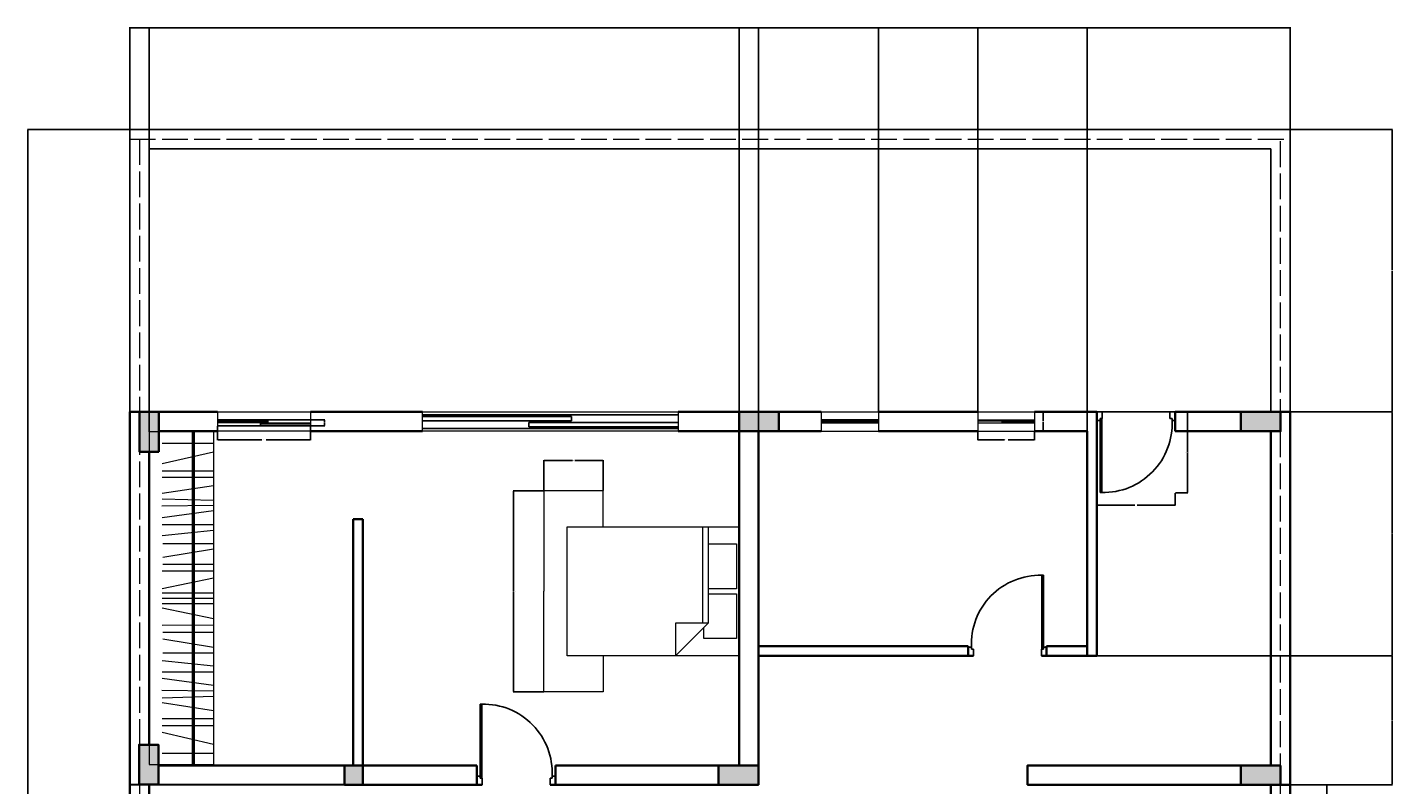
# Model space of a CAD drawing. Units: inches. Extents: x 2711 to 4246, y 540 to 1583.
# Tile 4 of 7: x 2716 to 3351, y 1230 to 1583. Entities that reach past the tile are written whole.
import ezdxf

# ---------------------------------------------------------------- set-up
doc = ezdxf.new("R2010")
doc.units = ezdxf.units.IN
doc.linetypes.add('ACAD_ISO02W100', pattern=[15, 12, -3])
for name, color, linetype, lineweight in [('A-ANNO-DIMS', 2, 'Continuous', 18), ('A-COLS', 210, 'Continuous', 35), ('A-COLS-PATT', 6, 'Continuous', 13), ('A-FLOR-CASE', 30, 'Continuous', 18), ('A-GLAZ', 4, 'Continuous', 18), ('A-WALL', 1, 'Continuous', 35), ('C-PROP-HIDN', 7, 'ACAD_ISO02W100', 13), ('C-PROP-WALL', 7, 'Continuous', 25), ('DOOR', 32, 'Continuous', 25), ('FURN', 30, 'Continuous', 18)]:
    doc.layers.add(name, color=color, linetype=linetype, lineweight=lineweight)
doc.layers.add('DARK', color=5, linetype='Continuous')
doc.styles.get("Standard").update_dxf_attribs({"font": 'arial.ttf'})
doc.dimstyles.get("Standard").update_dxf_attribs({"dimtxt": 0.18, "dimasz": 0.18, "dimexe": 0.18, "dimexo": 0.0625, "dimgap": 0.09, "dimtad": 0, "dimtih": 1, "dimtoh": 1, "dimdec": 4, "dimzin": 0, "dimdsep": 46, "dimtxsty": 'Standard', "dimcen": 0.09, "dimadec": 0, "dimazin": 0, "dimtfac": 1, "dimtdec": 4, "dimtofl": 0, "dimtmove": 0, "dimatfit": 3, "dimfxl": 1, "dimtolj": 1, "dimtzin": 0, "dimarcsym": 0})

# ---------------------------------------------------------------- blocks, each defined once
blk = doc.blocks.new('DOORS')
at = {"layer": 'DOOR'}
for p, q in [((-0.63, -0.36), (-0.63, -5.61)), ((-0.63, -5.61), (1.37, -5.61)), ((1.37, -5.61), (1.37, -4.36)), ((1.37, -4.36), (2.62, -4.36)), ((1.37, -5.61), (1.37, -49.61)), ((2.37, -49.61), (2.37, -4.36)), ((2.62, -4.36), (2.62, -0.36)), ((44.12, -4.36), (44.12, -0.36)), ((45.37, -4.36), (44.12, -4.36)), ((47.37, -5.61), (45.37, -5.61)), ((47.37, -0.36), (47.37, -5.61)), ((1.37, -49.61), (2.37, -49.61))]:
    blk.add_line(p, q, dxfattribs=at)
for centre, radius, start, end in [((3.41, -7.61), 42.01, 268.5852, 2.73188), ((38.76, -4.99), 6.64, 354.60229, 5.39771)]:
    blk.add_arc(centre, radius, start, end, dxfattribs=at)
blk = doc.blocks.new('DIPDASS')
at = {"layer": 'DARK'}
for p, q in [((0, 0), (109, 0)), ((0, -7.3), (109, -7.3))]:
    blk.add_line(p, q, dxfattribs=at)
at = {"layer": 'DOOR'}
for points in [[(0, -1.2), (56.3, -1.2), (58.8, -1.2), (58.8, -3.2), (56.3, -3.2), (0, -3.2)], [(109, -6.2), (52.7, -6.2), (50.2, -6.2), (50.2, -4.2), (52.7, -4.2), (109, -4.2)]]:
    blk.add_lwpolyline(points, dxfattribs=at)
blk = doc.blocks.new('DODO')
at = {"layer": 'DARK'}
for p, q in [((-118.96, 0), (0, 0)), ((-118.96, -6.4), (0, -6.4))]:
    blk.add_line(p, q, dxfattribs=at)
at = {"layer": 'DOOR'}
for p, q in [((-118.96, -0.88), (-49.49, -0.88)), ((-49.49, -2.88), (-118.96, -2.88)), ((0, -3.61), (-69.47, -3.61)), ((-69.47, -3.61), (-69.47, -5.61)), ((-69.47, -5.61), (0, -5.61)), ((-49.49, -0.88), (-49.49, -2.88))]:
    blk.add_line(p, q, dxfattribs=at)
blk = doc.blocks.new('Bed - Queen')
for p, q in [((0, -80.00003), (0, 0)), ((0, 0), (59.99999, 0)), ((59.99999, 0), (59.99999, -80.00003)), ((7.99999, -1.2), (28.79998, -1.2)), ((7.99999, -14.4), (7.99999, -1.2)), ((28.79998, -1.2), (28.79998, -14.4)), ((31.19999, -1.2), (51.99999, -1.2)), ((31.19999, -14.4), (31.19999, -1.2)), ((51.99999, -1.2), (51.99999, -16.4)), ((0, -14.4), (44.8, -14.4)), ((44.8, -16.8), (0, -16.8)), ((59.99999, -29.6), (44.8, -14.4)), ((44.8, -14.4), (44.8, -29.6)), ((51.99999, -16.4), (46.79936, -16.4)), ((44.8, -29.6), (59.99999, -29.6)), ((59.99999, -80.00003), (0, -80.00003))]:
    blk.add_line(p, q)
blk = doc.blocks.new('WARDROBE-LONG')
for p, q in [((29.95, 154.87), (0, 154.87)), ((0, 154.87), (0, 0)), ((20.07, 154.87), (20.07, 0)), ((20.11, 154.87), (20.11, 0)), ((20.16, 154.87), (20.16, 0)), ((20.2, 154.87), (20.2, 0)), ((20.23, 154.87), (20.23, 0)), ((20.29, 154.87), (20.29, 0)), ((20.35, 154.87), (20.35, 0)), ((20.41, 154.87), (20.41, 0)), ((20.45, 154.87), (20.45, 0)), ((20.49, 154.87), (20.49, 0)), ((20.55, 154.87), (20.55, 0)), ((20.6, 154.87), (20.6, 0)), ((20.66, 154.87), (20.66, 0)), ((20.73, 154.87), (20.73, 0)), ((20.78, 154.87), (20.78, 0)), ((20.83, 154.87), (20.83, 0)), ((20.87, 154.87), (20.87, 0)), ((20.92, 154.87), (20.92, 0)), ((20.92, 154.87), (20.92, 0)), ((29.95, 154.87), (29.95, 0)), ((6.03, 149.59), (29.95, 149.59)), ((29.95, 145.48), (6.03, 139.93)), ((6.03, 136.69), (29.95, 136.69)), ((29.95, 133.62), (6.03, 133.62)), ((29.95, 129.81), (6.03, 126.19)), ((6.03, 123.74), (29.95, 123.04)), ((29.95, 120.68), (5.93, 120.34)), ((29.95, 118.08), (6.01, 114.81)), ((6.01, 111.74), (29.95, 111.74)), ((29.95, 108.99), (6.01, 106.55)), ((6.38, 102.89), (29.95, 102.89)), ((29.95, 100.33), (6.38, 96.45)), ((29.95, 90.01), (6.01, 90.1)), ((6.38, 93.23), (29.95, 93.23)), ((6.01, 81.93), (29.95, 86.88)), ((6.01, 79.93), (29.95, 79.93)), ((6.01, 77.44), (29.95, 77.44)), ((6.01, 74.94), (29.95, 74.94)), ((6.01, 72.94), (29.95, 67.99)), ((29.95, 64.86), (6.01, 64.77)), ((6.38, 61.64), (29.95, 61.64)), ((29.95, 54.54), (6.38, 58.42)), ((6.38, 51.98), (29.95, 51.98)), ((29.95, 45.88), (6.01, 48.32)), ((6.01, 43.13), (29.95, 43.13)), ((29.95, 36.79), (6.01, 40.06)), ((29.95, 34.19), (5.93, 34.54)), ((6.03, 31.13), (29.95, 31.83)), ((29.95, 25.06), (6.03, 28.68)), ((29.95, 21.25), (6.03, 21.25)), ((6.03, 18.18), (29.95, 18.18)), ((29.95, 9.39), (6.03, 14.94)), ((0, 0), (29.95, 0)), ((6.03, 5.28), (29.95, 5.28))]:
    blk.add_line(p, q)
blk = doc.blocks.new('WIN-SLIDER-W01')
for p, q in [((0, 9), (26.39, 9)), ((0, 9), (0, 0)), ((26.39, 9), (26.39, 0)), ((0, 5.31), (26.39, 5.31)), ((0, 5.11), (15.65, 5.11)), ((15.65, 4.66), (0, 4.66)), ((0, 3.87), (26.39, 3.87)), ((0, 0), (26.39, 0)), ((26.39, 4.5), (11.15, 4.5)), ((11.15, 4.5), (11.15, 4.05)), ((11.15, 4.05), (26.39, 4.05)), ((15.65, 5.11), (15.65, 4.66))]:
    blk.add_line(p, q)
blk = doc.blocks.new('BED-BASE-QUEEN')
for p, q in [((27.64, 93.59), (0, 93.59)), ((0, 93.59), (0, 46.79)), ((27.64, 76.79), (27.64, 93.59)), ((0, 0), (0, 46.79)), ((27.64, 16.79), (27.64, 0)), ((27.64, 0), (0, 0))]:
    blk.add_line(p, q)
blk = doc.blocks.new('*D54')
at = {"layer": 'A-ANNO-DIMS', "color": 0, "lineweight": -2, "transparency": 16777216}
for p, q in [((3250.08, 1403.45), (3255.86, 1403.45)), ((3255.68, 1403.27), (3255.68, 1384.78)), ((3255.68, 1365.93), (3255.68, 1384.42)), ((3250.08, 1365.75), (3255.86, 1365.75))]:
    blk.add_line(p, q, dxfattribs=at)
at = {"layer": 'A-ANNO-DIMS', "color": 0, "transparency": 16777216}
for points in [[(3255.65, 1403.27), (3255.71, 1403.27), (3255.68, 1403.45)], [(3255.65, 1365.93), (3255.71, 1365.93), (3255.68, 1365.75)]]:
    blk.add_solid(points, dxfattribs=at)
at = {"layer": 'Defpoints', "color": 0, "transparency": 16777216}
for p in [(3250.02, 1403.45), (3255.68, 1403.45), (3250.02, 1365.75)]:
    blk.add_point(p, dxfattribs=at)
at = {"layer": 'A-ANNO-DIMS', "color": 0, "transparency": 16777216, "insert": (3255.68, 1384.6), "char_height": 0.18, "attachment_point": 5}
blk.add_mtext('\\A1;DOOR 38 TYP.', dxfattribs=at)
blk = doc.blocks.new('*D55')
at = {"layer": 'A-ANNO-DIMS', "color": 0, "lineweight": -2, "transparency": 16777216}
for p, q in [((3213.5, 1365.69), (3213.5, 1359.92)), ((3213.68, 1360.1), (3231.23, 1360.1)), ((3249.84, 1360.1), (3232.29, 1360.1)), ((3250.02, 1365.69), (3250.02, 1359.92))]:
    blk.add_line(p, q, dxfattribs=at)
at = {"layer": 'A-ANNO-DIMS', "color": 0, "transparency": 16777216}
for points in [[(3213.68, 1360.13), (3213.68, 1360.07), (3213.5, 1360.1)], [(3249.84, 1360.13), (3249.84, 1360.07), (3250.02, 1360.1)]]:
    blk.add_solid(points, dxfattribs=at)
at = {"layer": 'Defpoints', "color": 0, "transparency": 16777216}
for p in [(3213.5, 1365.75), (3250.02, 1365.75), (3250.02, 1360.1)]:
    blk.add_point(p, dxfattribs=at)
at = {"layer": 'A-ANNO-DIMS', "color": 0, "transparency": 16777216, "insert": (3231.76, 1360.1), "char_height": 0.18, "attachment_point": 5}
blk.add_mtext('\\A1;37 TYP.', dxfattribs=at)
blk = doc.blocks.new('*D64')
at = {"layer": 'A-ANNO-DIMS', "color": 0, "lineweight": -2, "transparency": 16777216}
for p, q in [((2804.38, 1396.9), (2804.38, 1390.29)), ((2847.61, 1396.9), (2847.61, 1390.29)), ((2804.56, 1390.47), (2824.98, 1390.47)), ((2847.43, 1390.47), (2827.01, 1390.47))]:
    blk.add_line(p, q, dxfattribs=at)
at = {"layer": 'A-ANNO-DIMS', "color": 0, "transparency": 16777216}
for points in [[(2804.56, 1390.5), (2804.56, 1390.44), (2804.38, 1390.47)], [(2847.43, 1390.5), (2847.43, 1390.44), (2847.61, 1390.47)]]:
    blk.add_solid(points, dxfattribs=at)
at = {"layer": 'Defpoints', "color": 0, "transparency": 16777216}
for p in [(2804.38, 1396.96), (2847.61, 1396.96), (2847.61, 1390.47)]:
    blk.add_point(p, dxfattribs=at)
at = {"layer": 'A-ANNO-DIMS', "color": 0, "transparency": 16777216, "insert": (2826, 1390.47), "char_height": 0.18, "attachment_point": 5}
blk.add_mtext('\\A1;SLIDER 43 TYP.', dxfattribs=at)
blk = doc.blocks.new('*D65')
at = {"layer": 'A-ANNO-DIMS', "color": 0, "lineweight": -2, "transparency": 16777216}
for p, q in [((2847.68, 1399.83), (2854.28, 1399.83)), ((2854.1, 1399.65), (2854.1, 1398.58)), ((2854.1, 1397.14), (2854.1, 1398.21)), ((2847.68, 1396.96), (2854.28, 1396.96))]:
    blk.add_line(p, q, dxfattribs=at)
at = {"layer": 'A-ANNO-DIMS', "color": 0, "transparency": 16777216}
for points in [[(2854.07, 1399.65), (2854.13, 1399.65), (2854.1, 1399.83)], [(2854.07, 1397.14), (2854.13, 1397.14), (2854.1, 1396.96)]]:
    blk.add_solid(points, dxfattribs=at)
at = {"layer": 'Defpoints', "color": 0, "transparency": 16777216}
for p in [(2847.61, 1399.83), (2854.1, 1399.83), (2847.61, 1396.96)]:
    blk.add_point(p, dxfattribs=at)
at = {"layer": 'A-ANNO-DIMS', "color": 0, "transparency": 16777216, "insert": (2854.1, 1398.4), "char_height": 0.18, "attachment_point": 5}
blk.add_mtext('\\A1;3 TYP.', dxfattribs=at)
blk = doc.blocks.new('*D72')
at = {"layer": 'A-ANNO-DIMS', "color": 0, "lineweight": -2, "transparency": 16777216}
for p, q in [((2956.1, 1366.79), (2941.95, 1366.79)), ((2942.13, 1366.61), (2942.13, 1320.18)), ((2942.13, 1273.39), (2942.13, 1319.82)), ((2956.1, 1273.21), (2941.95, 1273.21))]:
    blk.add_line(p, q, dxfattribs=at)
at = {"layer": 'A-ANNO-DIMS', "color": 0, "transparency": 16777216}
for points in [[(2942.1, 1366.61), (2942.16, 1366.61), (2942.13, 1366.79)], [(2942.1, 1273.39), (2942.16, 1273.39), (2942.13, 1273.21)]]:
    blk.add_solid(points, dxfattribs=at)
at = {"layer": 'Defpoints', "color": 0, "transparency": 16777216}
for p in [(2942.13, 1366.79), (2956.17, 1366.79), (2956.17, 1273.21)]:
    blk.add_point(p, dxfattribs=at)
at = {"layer": 'A-ANNO-DIMS', "color": 0, "transparency": 16777216, "insert": (2942.13, 1320), "char_height": 0.18, "attachment_point": 5}
blk.add_mtext('\\A1;BED BASE 94 TYP.', dxfattribs=at)
blk = doc.blocks.new('*D73')
at = {"layer": 'A-ANNO-DIMS', "color": 0, "lineweight": -2, "transparency": 16777216}
for p, q in [((2956.17, 1366.86), (2956.17, 1381.01)), ((2956.35, 1380.83), (2969.46, 1380.83)), ((2983.63, 1380.83), (2970.52, 1380.83)), ((2983.81, 1366.86), (2983.81, 1381.01))]:
    blk.add_line(p, q, dxfattribs=at)
at = {"layer": 'A-ANNO-DIMS', "color": 0, "transparency": 16777216}
for points in [[(2956.35, 1380.86), (2956.35, 1380.8), (2956.17, 1380.83)], [(2983.63, 1380.86), (2983.63, 1380.8), (2983.81, 1380.83)]]:
    blk.add_solid(points, dxfattribs=at)
at = {"layer": 'Defpoints', "color": 0, "transparency": 16777216}
for p in [(2983.81, 1380.83), (2956.17, 1366.79), (2983.81, 1366.79)]:
    blk.add_point(p, dxfattribs=at)
at = {"layer": 'A-ANNO-DIMS', "color": 0, "transparency": 16777216, "insert": (2969.99, 1380.83), "char_height": 0.18, "attachment_point": 5}
blk.add_mtext('\\A1;28 TYP.', dxfattribs=at)
blk = doc.blocks.new('*D82')
at = {"layer": 'A-ANNO-DIMS', "color": 0, "lineweight": -2, "transparency": 16777216}
for p, q in [((3294.56, 1229.95), (3320.78, 1229.95)), ((3320.6, 1229.77), (3320.6, 1143.13)), ((3320.6, 1056.12), (3320.6, 1142.76)), ((3294.56, 1055.94), (3320.78, 1055.94))]:
    blk.add_line(p, q, dxfattribs=at)
at = {"layer": 'A-ANNO-DIMS', "color": 0, "transparency": 16777216}
for points in [[(3320.57, 1229.77), (3320.63, 1229.77), (3320.6, 1229.95)], [(3320.57, 1056.12), (3320.63, 1056.12), (3320.6, 1055.94)]]:
    blk.add_solid(points, dxfattribs=at)
at = {"layer": 'Defpoints', "color": 0, "transparency": 16777216}
for p in [(3294.5, 1229.95), (3320.6, 1229.95), (3294.5, 1055.94)]:
    blk.add_point(p, dxfattribs=at)
at = {"layer": 'A-ANNO-DIMS', "color": 0, "transparency": 16777216, "insert": (3320.6, 1142.95), "char_height": 0.18, "attachment_point": 5}
blk.add_mtext('\\A1;RETURN STAIR 174 TYP.', dxfattribs=at)
blk = doc.blocks.new('*D86')
at = {"layer": 'A-ANNO-DIMS', "color": 0, "lineweight": -2, "transparency": 16777216}
for p, q in [((3158.15, 1394.39), (3158.15, 1390.31)), ((3184.54, 1394.39), (3184.54, 1390.31)), ((3158.33, 1390.49), (3170.52, 1390.49)), ((3184.36, 1390.49), (3172.17, 1390.49))]:
    blk.add_line(p, q, dxfattribs=at)
at = {"layer": 'A-ANNO-DIMS', "color": 0, "transparency": 16777216}
for points in [[(3158.33, 1390.52), (3158.33, 1390.46), (3158.15, 1390.49)], [(3184.36, 1390.52), (3184.36, 1390.46), (3184.54, 1390.49)]]:
    blk.add_solid(points, dxfattribs=at)
at = {"layer": 'Defpoints', "color": 0, "transparency": 16777216}
for p in [(3158.15, 1394.45), (3184.54, 1394.45), (3184.54, 1390.49)]:
    blk.add_point(p, dxfattribs=at)
at = {"layer": 'A-ANNO-DIMS', "color": 0, "transparency": 16777216, "insert": (3171.35, 1390.49), "char_height": 0.18, "attachment_point": 5}
blk.add_mtext('\\A1;W01 26 TYP.', dxfattribs=at)
blk = doc.blocks.new('*D87')
at = {"layer": 'A-ANNO-DIMS', "color": 0, "lineweight": -2, "transparency": 16777216}
for p, q in [((3184.6, 1403.45), (3188.68, 1403.45)), ((3188.5, 1403.27), (3188.5, 1399.13)), ((3188.5, 1394.63), (3188.5, 1398.77)), ((3184.6, 1394.45), (3188.68, 1394.45))]:
    blk.add_line(p, q, dxfattribs=at)
at = {"layer": 'A-ANNO-DIMS', "color": 0, "transparency": 16777216}
for points in [[(3188.47, 1403.27), (3188.53, 1403.27), (3188.5, 1403.45)], [(3188.47, 1394.63), (3188.53, 1394.63), (3188.5, 1394.45)]]:
    blk.add_solid(points, dxfattribs=at)
at = {"layer": 'Defpoints', "color": 0, "transparency": 16777216}
for p in [(3184.54, 1403.45), (3188.5, 1403.45), (3184.54, 1394.45)]:
    blk.add_point(p, dxfattribs=at)
at = {"layer": 'A-ANNO-DIMS', "color": 0, "transparency": 16777216, "insert": (3188.5, 1398.95), "char_height": 0.18, "attachment_point": 5}
blk.add_mtext('\\A1;9 TYP.', dxfattribs=at)
blk = doc.blocks.new('*D94')
at = {"layer": 'A-ANNO-DIMS', "color": 0, "lineweight": -2, "transparency": 16777216}
for p, q in [((2763.5, 1535.01), (2763.5, 1582.51)), ((2763.68, 1582.33), (3033.21, 1582.33)), ((3303.32, 1582.33), (3033.78, 1582.33)), ((3303.5, 1535.01), (3303.5, 1582.51))]:
    blk.add_line(p, q, dxfattribs=at)
at = {"layer": 'A-ANNO-DIMS', "color": 0, "transparency": 16777216}
for points in [[(2763.68, 1582.36), (2763.68, 1582.3), (2763.5, 1582.33)], [(3303.32, 1582.36), (3303.32, 1582.3), (3303.5, 1582.33)]]:
    blk.add_solid(points, dxfattribs=at)
at = {"layer": 'Defpoints', "color": 0, "transparency": 16777216}
for p in [(3303.5, 1582.33), (2763.5, 1534.95), (3303.5, 1534.95)]:
    blk.add_point(p, dxfattribs=at)
at = {"layer": 'A-ANNO-DIMS', "color": 0, "transparency": 16777216, "insert": (3033.5, 1582.33), "char_height": 0.18, "attachment_point": 5}
blk.add_mtext('\\A1;540', dxfattribs=at)
blk = doc.blocks.new('*D95')
at = {"layer": 'A-ANNO-DIMS', "color": 0, "lineweight": -2, "transparency": 16777216}
for p, q in [((2763.43, 1534.95), (2715.94, 1534.95)), ((2716.12, 1534.77), (2716.12, 1061.38)), ((2716.12, 587.63), (2716.12, 1061.02)), ((2763.43, 587.45), (2715.94, 587.45))]:
    blk.add_line(p, q, dxfattribs=at)
at = {"layer": 'A-ANNO-DIMS', "color": 0, "transparency": 16777216}
for points in [[(2716.09, 1534.77), (2716.15, 1534.77), (2716.12, 1534.95)], [(2716.09, 587.63), (2716.15, 587.63), (2716.12, 587.45)]]:
    blk.add_solid(points, dxfattribs=at)
at = {"layer": 'Defpoints', "color": 0, "transparency": 16777216}
for p in [(2716.12, 1534.95), (2763.5, 1534.95), (2763.5, 587.45)]:
    blk.add_point(p, dxfattribs=at)
at = {"layer": 'A-ANNO-DIMS', "color": 0, "transparency": 16777216, "insert": (2716.12, 1061.2), "char_height": 0.18, "attachment_point": 5}
blk.add_mtext('\\A1;947.5', dxfattribs=at)
blk = doc.blocks.new('*D101')
at = {"layer": 'A-ANNO-DIMS', "color": 0, "lineweight": -2, "transparency": 16777216}
for p, q in [((3209.06, 1289.95), (3351.05, 1289.95)), ((3350.87, 1289.77), (3350.87, 1260.13)), ((3350.87, 1230.13), (3350.87, 1259.77)), ((3299.06, 1229.95), (3351.05, 1229.95))]:
    blk.add_line(p, q, dxfattribs=at)
at = {"layer": 'A-ANNO-DIMS', "color": 0, "transparency": 16777216}
for points in [[(3350.84, 1289.77), (3350.9, 1289.77), (3350.87, 1289.95)], [(3350.84, 1230.13), (3350.9, 1230.13), (3350.87, 1229.95)]]:
    blk.add_solid(points, dxfattribs=at)
at = {"layer": 'Defpoints', "color": 0, "transparency": 16777216}
for p in [(3209, 1289.95), (3350.87, 1289.95), (3299, 1229.95)]:
    blk.add_point(p, dxfattribs=at)
at = {"layer": 'A-ANNO-DIMS', "color": 0, "transparency": 16777216, "insert": (3350.87, 1259.95), "char_height": 0.18, "attachment_point": 5}
blk.add_mtext('\\A1;60', dxfattribs=at)
blk = doc.blocks.new('*D102')
at = {"layer": 'A-ANNO-DIMS', "color": 0, "lineweight": -2, "transparency": 16777216}
for p, q in [((3299.06, 1403.45), (3351.05, 1403.45)), ((3350.87, 1403.27), (3350.87, 1346.88)), ((3350.87, 1290.13), (3350.87, 1346.52)), ((3209.06, 1289.95), (3351.05, 1289.95))]:
    blk.add_line(p, q, dxfattribs=at)
at = {"layer": 'A-ANNO-DIMS', "color": 0, "transparency": 16777216}
for points in [[(3350.84, 1403.27), (3350.9, 1403.27), (3350.87, 1403.45)], [(3350.84, 1290.13), (3350.9, 1290.13), (3350.87, 1289.95)]]:
    blk.add_solid(points, dxfattribs=at)
at = {"layer": 'Defpoints', "color": 0, "transparency": 16777216}
for p in [(3299, 1403.45), (3350.87, 1403.45), (3209, 1289.95)]:
    blk.add_point(p, dxfattribs=at)
at = {"layer": 'A-ANNO-DIMS', "color": 0, "transparency": 16777216, "insert": (3350.87, 1346.7), "char_height": 0.18, "attachment_point": 5}
blk.add_mtext('\\A1;113.5', dxfattribs=at)
blk = doc.blocks.new('*D103')
at = {"layer": 'A-ANNO-DIMS', "color": 0, "lineweight": -2, "transparency": 16777216}
for p, q in [((3303.56, 1534.95), (3351.05, 1534.95)), ((3350.87, 1534.77), (3350.87, 1469.38)), ((3350.87, 1403.63), (3350.87, 1469.02)), ((3299.06, 1403.45), (3351.05, 1403.45))]:
    blk.add_line(p, q, dxfattribs=at)
at = {"layer": 'A-ANNO-DIMS', "color": 0, "transparency": 16777216}
for points in [[(3350.84, 1534.77), (3350.9, 1534.77), (3350.87, 1534.95)], [(3350.84, 1403.63), (3350.9, 1403.63), (3350.87, 1403.45)]]:
    blk.add_solid(points, dxfattribs=at)
at = {"layer": 'Defpoints', "color": 0, "transparency": 16777216}
for p in [(3303.5, 1534.95), (3350.87, 1534.95), (3299, 1403.45)]:
    blk.add_point(p, dxfattribs=at)
at = {"layer": 'A-ANNO-DIMS', "color": 0, "transparency": 16777216, "insert": (3350.87, 1469.2), "char_height": 0.18, "attachment_point": 5}
blk.add_mtext('\\A1;131.5', dxfattribs=at)
blk = doc.blocks.new('*D113')
at = {"layer": 'A-ANNO-DIMS', "color": 0, "lineweight": -2, "transparency": 16777216}
for p, q in [((2772.5, 1394.24), (2772.5, 1582.51)), ((2772.68, 1582.33), (2909.35, 1582.33)), ((3046.82, 1582.33), (2910.14, 1582.33)), ((3047, 1394.51), (3047, 1582.51))]:
    blk.add_line(p, q, dxfattribs=at)
at = {"layer": 'A-ANNO-DIMS', "color": 0, "transparency": 16777216}
for points in [[(2772.68, 1582.36), (2772.68, 1582.3), (2772.5, 1582.33)], [(3046.82, 1582.36), (3046.82, 1582.3), (3047, 1582.33)]]:
    blk.add_solid(points, dxfattribs=at)
at = {"layer": 'Defpoints', "color": 0, "transparency": 16777216}
for p in [(3047, 1582.33), (2772.5, 1394.18), (3047, 1394.45)]:
    blk.add_point(p, dxfattribs=at)
at = {"layer": 'A-ANNO-DIMS', "color": 0, "transparency": 16777216, "insert": (2909.75, 1582.33), "char_height": 0.18, "attachment_point": 5}
blk.add_mtext('\\A1;274.5', dxfattribs=at)
blk = doc.blocks.new('*D114')
at = {"layer": 'A-ANNO-DIMS', "color": 0, "lineweight": -2, "transparency": 16777216}
for p, q in [((3056, 1394.51), (3056, 1582.51)), ((3056.18, 1582.33), (3132.22, 1582.33)), ((3208.82, 1582.33), (3132.78, 1582.33)), ((3209, 1394.51), (3209, 1582.51))]:
    blk.add_line(p, q, dxfattribs=at)
at = {"layer": 'A-ANNO-DIMS', "color": 0, "transparency": 16777216}
for points in [[(3056.18, 1582.36), (3056.18, 1582.3), (3056, 1582.33)], [(3208.82, 1582.36), (3208.82, 1582.3), (3209, 1582.33)]]:
    blk.add_solid(points, dxfattribs=at)
at = {"layer": 'Defpoints', "color": 0, "transparency": 16777216}
for p in [(3209, 1582.33), (3056, 1394.45), (3209, 1394.45)]:
    blk.add_point(p, dxfattribs=at)
at = {"layer": 'A-ANNO-DIMS', "color": 0, "transparency": 16777216, "insert": (3132.5, 1582.33), "char_height": 0.18, "attachment_point": 5}
blk.add_mtext('\\A1;153', dxfattribs=at)
blk = doc.blocks.new('*D118')
at = {"layer": 'A-ANNO-DIMS', "color": 0, "lineweight": -2, "transparency": 16777216}
for p, q in [((3111.96, 1403.51), (3111.96, 1582.51)), ((3112.14, 1582.33), (3134.66, 1582.33)), ((3157.97, 1582.33), (3135.45, 1582.33)), ((3158.15, 1403.51), (3158.15, 1582.51))]:
    blk.add_line(p, q, dxfattribs=at)
at = {"layer": 'A-ANNO-DIMS', "color": 0, "transparency": 16777216}
for points in [[(3112.14, 1582.36), (3112.14, 1582.3), (3111.96, 1582.33)], [(3157.97, 1582.36), (3157.97, 1582.3), (3158.15, 1582.33)]]:
    blk.add_solid(points, dxfattribs=at)
at = {"layer": 'Defpoints', "color": 0, "transparency": 16777216}
for p in [(3158.15, 1582.33), (3111.96, 1403.45), (3158.15, 1403.45)]:
    blk.add_point(p, dxfattribs=at)
at = {"layer": 'A-ANNO-DIMS', "color": 0, "transparency": 16777216, "insert": (3135.06, 1582.33), "char_height": 0.18, "attachment_point": 5}
blk.add_mtext('\\A1;46.19', dxfattribs=at)

msp = doc.modelspace()

# ---------------------------------------------------------------- hatches: boundary and pattern name
at = {"layer": 'A-COLS-PATT'}
h = msp.add_hatch(color=256, dxfattribs=at)
h.dxf.hatch_style = 1
h.paths.add_polyline_path([(2767.9955, 1384.9055), (2776.9955, 1384.9055), (2776.9955, 1403.4493), (2767.9955, 1403.4493)])
h.paths.add_polyline_path([(3065.5392, 1394.4493), (3065.5392, 1403.4493), (3046.9955, 1403.4493), (3046.9955, 1394.4493)])
h.paths.add_polyline_path([(3298.9955, 1394.4493), (3298.9955, 1403.4493), (3280.4517, 1403.4493), (3280.4517, 1394.4493)])
h.paths.add_polyline_path([(2767.8485, 1230.0438), (2776.8485, 1230.0353), (2776.8485, 1248.5791), (2767.8485, 1248.5791)])
h.paths.add_polyline_path([(2871.9955, 1229.9493), (2871.9955, 1238.9493), (2863.4422, 1238.9493), (2863.4422, 1229.9531), (2867.4955, 1229.9493)])
h.paths.add_polyline_path([(3055.9955, 1229.9493), (3055.9955, 1238.9493), (3037.4517, 1238.9493), (3037.4517, 1229.9493)])
h.paths.add_polyline_path([(3298.9955, 1229.9493), (3298.9955, 1238.9493), (3280.4517, 1238.9493), (3280.4517, 1229.9493)])
h.paths.add_polyline_path([(2776.8485, 1056.0394), (2767.8485, 1056.0394), (2767.8485, 1037.4957), (2776.8485, 1037.4957)])
h.paths.add_polyline_path([(2973.0214, 1041.7894), (2973.0214, 1037.4957), (2982.0148, 1037.4957), (2982.0148, 1056.0394), (2973.0148, 1056.0394), (2973.0148, 1052.2894), (2973.0214, 1052.2894), (2973.0214, 1047.0394)])
h.paths.add_polyline_path([(3063.0214, 1037.4957), (3063.0214, 1056.0394), (3054.0214, 1056.0394), (3054.0214, 1037.4957)])
h.paths.add_polyline_path([(3294.4955, 1046.9493), (3298.9955, 1046.9493), (3298.9955, 1055.9413), (3280.4517, 1055.9413), (3280.4517, 1046.9493)])
h.paths.add_polyline_path([(2982.0214, 924.0394), (2973.0214, 924.0394), (2973.0214, 905.4957), (2982.0214, 905.4957)])
h.paths.add_polyline_path([(3054.0214, 905.4957), (3063.0214, 905.4957), (3063.0214, 924.0394), (3054.0214, 924.0394)])
h.paths.add_polyline_path([(3216.0214, 905.7675), (3216.0214, 914.7675), (3197.4776, 914.7675), (3197.4776, 905.7675)])
h.paths.add_polyline_path([(2776.8485, 842.8947), (2776.8485, 861.4385), (2767.8485, 861.4385), (2767.8485, 842.8947)])
h.paths.add_polyline_path([(3294.4955, 824.7675), (3298.9955, 824.7498), (3298.9955, 833.7498), (3280.4517, 833.7498), (3280.4517, 824.7675)])
h.paths.add_polyline_path([(2793.6045, 587.4493), (2793.6045, 599.3563), (2767.9955, 599.3563), (2767.9955, 587.4493)])
h.paths.add_polyline_path([(2922.1577, 587.4493), (2922.1577, 596.4493), (2913.6045, 596.4493), (2913.6045, 587.4493)])
h.paths.add_polyline_path([(2995.7668, 587.4493), (2995.7668, 599.3563), (2970.1577, 599.3563), (2970.1577, 587.4493)])

# ---------------------------------------------------------------- linework, layer by layer
at = {"layer": 'A-COLS'}
for points in [[(2776.9955, 1384.9055), (2776.9955, 1403.4493), (2767.9955, 1403.4493), (2767.9955, 1384.9055)], [(3065.5392, 1403.4493), (3046.9955, 1403.4493), (3046.9955, 1394.4493), (3065.5392, 1394.4493)], [(3298.9955, 1403.4493), (3280.4517, 1403.4493), (3280.4517, 1394.4493), (3298.9955, 1394.4493)], [(2776.8485, 1230.0353), (2776.8485, 1248.5791), (2767.8485, 1248.5791), (2767.8485, 1230.0353)], [(2863.4422, 1229.9493), (2871.9955, 1229.9493), (2871.9955, 1238.9493), (2863.4422, 1238.9493)], [(3055.9955, 1238.9493), (3037.4517, 1238.9493), (3037.4517, 1229.9493), (3055.9955, 1229.9493)], [(3298.9955, 1238.9493), (3280.4517, 1238.9493), (3280.4517, 1229.9493), (3298.9955, 1229.9493)]]:
    msp.add_lwpolyline(points, close=True, dxfattribs=at)
at = {"layer": 'A-GLAZ'}
for p, q in [((2804.3779, 1403.4493), (2804.3779, 1394.4493)), ((2804.3779, 1403.4493), (2847.6139, 1403.4493)), ((2847.6139, 1403.4493), (2847.6139, 1394.4493)), ((2899.6522, 1394.4493), (2899.6522, 1403.4493)), ((2899.6522, 1403.4493), (3018.6125, 1403.4493)), ((3018.6125, 1403.4493), (3018.6125, 1394.4493)), ((3085.1509, 1403.4493), (3085.1509, 1394.4493)), ((3085.1509, 1403.4493), (3111.9592, 1403.4493)), ((3111.9592, 1403.4493), (3111.9592, 1394.4493)), ((2847.6139, 1394.4493), (2804.3779, 1394.4493)), ((3018.6125, 1394.4493), (2899.6522, 1394.4493)), ((3085.1509, 1394.4493), (3111.9592, 1394.4493))]:
    msp.add_line(p, q, dxfattribs=at)
at = {"layer": 'A-WALL'}
for p, q in [((2763.4955, 1403.4493), (2763.4955, 1230.048)), ((2804.3779, 1403.4493), (2763.4955, 1403.4493)), ((2899.6522, 1403.4493), (2847.6139, 1403.4493)), ((3046.9955, 1403.4493), (3018.6125, 1403.4493)), ((3055.9955, 1403.4493), (3046.9955, 1403.4493)), ((3046.9955, 1403.4493), (3046.9955, 1238.9493)), ((3085.1509, 1403.4493), (3055.9955, 1403.4493)), ((3158.1528, 1403.4493), (3111.9592, 1403.4493)), ((3208.9955, 1403.4493), (3184.5415, 1403.4493)), ((3213.4955, 1403.4493), (3208.9955, 1403.4493)), ((3213.4955, 1403.4493), (3213.4955, 1294.4493)), ((3294.4955, 1403.4493), (3250.0208, 1403.4493)), ((3250.0208, 1403.4493), (3250.0208, 1394.4493)), ((3303.4955, 1403.4493), (3294.4955, 1403.4493)), ((3303.4955, 1229.9493), (3303.4955, 1403.4493)), ((2776.9955, 1394.4493), (2804.3779, 1394.4493)), ((2847.6139, 1394.4493), (2899.6522, 1394.4493)), ((2856.5462, 1394.4493), (2899.6522, 1394.4493)), ((3018.6125, 1394.4493), (3046.9955, 1394.4493)), ((3055.9955, 1394.4493), (3046.9955, 1394.4493)), ((3055.9955, 1394.4493), (3055.9955, 1289.9493)), ((3085.1509, 1394.4493), (3055.9955, 1394.4493)), ((3158.1528, 1394.4493), (3111.9592, 1394.4493)), ((3208.9955, 1394.4493), (3184.5415, 1394.4493)), ((3208.9955, 1394.4493), (3208.9955, 1289.9493)), ((3250.0208, 1394.4493), (3294.4955, 1394.4493)), ((3294.4955, 1394.4493), (3294.4955, 1238.9493)), ((2772.4955, 1248.5791), (2772.4955, 1384.9055)), ((2772.4955, 1248.5791), (2772.4955, 1384.9055)), ((2871.9955, 1353.5477), (2867.4955, 1353.5477)), ((2867.4955, 1353.5477), (2867.4955, 1238.9493)), ((2871.9955, 1238.9493), (2871.9955, 1353.5477)), ((3153.6294, 1294.4493), (3055.9955, 1294.4493)), ((3055.9955, 1289.9493), (3156.1025, 1289.9493)), ((3055.9955, 1289.9493), (3055.9955, 1238.9493)), ((3153.6294, 1294.4493), (3153.6294, 1289.9493)), ((3187.6817, 1289.9493), (3213.4955, 1289.9493)), ((3208.9955, 1294.4493), (3190.1548, 1294.4493)), ((3190.1548, 1294.4493), (3190.1548, 1289.9493)), ((3208.9955, 1289.9493), (3208.9955, 1294.4493)), ((3213.4955, 1294.4493), (3213.4955, 1289.9493)), ((2867.4955, 1238.9493), (2776.8485, 1238.9493)), ((2867.4955, 1238.9493), (2871.9955, 1238.9493)), ((2925.0214, 1238.9493), (2871.9955, 1238.9493)), ((2925.0214, 1238.9493), (2925.0214, 1229.9493)), ((3055.9955, 1238.9493), (2961.5467, 1238.9493)), ((2961.5467, 1229.9493), (2961.5467, 1238.9493)), ((3055.9955, 1238.9493), (3055.9955, 1229.9493)), ((2763.4955, 1230.048), (2867.4955, 1229.9493)), ((2763.4955, 1047.0394), (2763.4955, 1230.048)), ((2772.4955, 1230.0394), (2772.4955, 1056.0394)), ((2772.4955, 1056.0394), (2772.4955, 1230.0394)), ((2927.4945, 1229.9493), (2867.4955, 1229.9493)), ((3055.9955, 1229.9493), (2959.0737, 1229.9493)), ((3294.4955, 1229.9493), (3294.4955, 1055.9413)), ((3294.4955, 1229.9493), (3294.4955, 1055.9493)), ((3298.9955, 1229.9493), (3303.4955, 1229.9493)), ((3303.4955, 1046.9493), (3303.4955, 1229.9493))]:
    msp.add_line(p, q, dxfattribs=at)
msp.add_lwpolyline([(3294.4955, 1238.9493), (3213.4955, 1238.9493), (3181.2888, 1238.9493), (3181.2888, 1229.9493), (3213.4955, 1229.9493), (3294.4955, 1229.9493)], dxfattribs=at)
at = {"layer": 'C-PROP-HIDN'}
for p, q in [((2763.4955, 1530.4493), (3303.4955, 1530.4493)), ((2767.9955, 1530.4493), (2767.9955, 1248.5791)), ((3298.9955, 587.4493), (3298.9955, 1530.4493)), ((2767.9955, 1230.0353), (2767.9955, 1056.0394))]:
    msp.add_line(p, q, dxfattribs=at)
at = {"layer": 'C-PROP-WALL'}
for p, q in [((2763.4955, 1534.9493), (2767.9955, 1534.9493)), ((2763.4955, 1530.4493), (2763.4955, 1534.9493)), ((2767.9955, 1534.9493), (3298.9955, 1534.9493)), ((3298.9955, 1534.9493), (3303.4955, 1534.9493)), ((3303.4955, 1534.9493), (3303.4955, 1530.4493)), ((2763.4955, 587.4493), (2763.4955, 1530.4493)), ((2772.4955, 1525.9493), (3294.4955, 1525.9493)), ((2772.4955, 1403.4493), (2772.4955, 1525.9493)), ((3294.4955, 1525.9493), (3294.4955, 1403.4493)), ((3303.4955, 1530.4493), (3303.4955, 587.4493))]:
    msp.add_line(p, q, dxfattribs=at)
at = {"layer": 'DOOR'}
msp.add_line((3213.4955, 1403.4493), (3250.0208, 1403.4493), dxfattribs=at)

# ---------------------------------------------------------------- block references
at = {"layer": 'A-FLOR-CASE'}
msp.add_blockref('WARDROBE-LONG', (2772.495, 1239.307), dxfattribs=at)
at = {"layer": 'A-GLAZ'}
for name, p, xscale, yscale, zscale in [('DIPDASS', (2804.3779, 1399.8345), 0.3965780416186425, 0.3965780416186425, 0.3965780416186425), ('DODO', (3111.9592, 1399.7619), 0.2253547321596577, 0.2253547321596577, 0.2253547321596577)]:
    msp.add_blockref(name, p, dxfattribs=dict(at, xscale=xscale, yscale=yscale, zscale=zscale))
for name, p in [('DODO', (3018.6125, 1402.1484)), ('WIN-SLIDER-W01', (3158.153, 1394.449))]:
    msp.add_blockref(name, p, dxfattribs=at)
at = {"layer": 'DOOR', "xscale": 0.7609445437706661, "yscale": 0.7609445437706661, "zscale": 0.7609445437706661}
msp.add_blockref('DOORS', (3213.9726, 1403.7248), dxfattribs=at)
at = {"layer": 'DOOR', "yscale": 0.7609445437706661, "zscale": 0.7609445437706661, "rotation": 180}
for p, xscale in [((3189.6776, 1289.6738), 0.7609445437706661), ((2925.4985, 1229.6738), -0.7609445437706661)]:
    msp.add_blockref('DOORS', p, dxfattribs=dict(at, xscale=xscale))
at = {"layer": 'FURN'}
msp.add_blockref('BED-BASE-QUEEN', (2956.166, 1273.205), dxfattribs=at)
at = {"layer": 'FURN', "rotation": 270}
msp.add_blockref('Bed - Queen', (3046.9955, 1349.9992), dxfattribs=at)

# ---------------------------------------------------------------- dimensions: what is measured, and where the dimension line sits
at = {"layer": 'A-ANNO-DIMS'}
for base, p1, p2, override, picture, middle in [((3303.4955, 1582.3263), (2763.4955, 1534.9493), (3303.4955, 1534.9493), {"dimdec": 0, "dimlfac": 1, "dimrnd": 0, "dimzin": 0, "dimdsep": 46, "dimlunit": 2}, '*D94', (3033.4955, 1582.3263)), ((3046.9955, 1582.3263), (2772.4955, 1394.1774), (3046.9955, 1394.4493), {"dimdec": 1, "dimlfac": 1, "dimrnd": 0, "dimzin": 0, "dimdsep": 46, "dimlunit": 2}, '*D113', (2909.7455, 1582.3263)), ((3208.9955, 1582.3263), (3055.9955, 1394.4493), (3208.9955, 1394.4493), {"dimdec": 0, "dimlfac": 1, "dimrnd": 0, "dimzin": 0, "dimdsep": 46, "dimlunit": 2}, '*D114', (3132.4955, 1582.3263)), ((3158.1528, 1582.3263), (3111.9592, 1403.4493), (3158.1528, 1403.4493), {"dimdec": 2, "dimlfac": 1, "dimrnd": 0, "dimzin": 0, "dimdsep": 46, "dimlunit": 2}, '*D118', (3135.056, 1582.3263))]:
    dim = msp.add_linear_dim(base=base, p1=p1, p2=p2, dimstyle='Standard', override=override, dxfattribs=at)
    dim.commit()
    dim.dimension.update_dxf_attribs({"geometry": picture, "text_midpoint": middle})
for base, p1, p2, override, picture, middle in [((2716.1185, 1534.9493), (2763.4955, 587.4493), (2763.4955, 1534.9493), {"dimdec": 1, "dimlfac": 1, "dimrnd": 0, "dimzin": 0, "dimdsep": 46, "dimlunit": 2}, '*D95', (2716.1185, 1061.1993)), ((3350.8725, 1534.9493), (3298.9955, 1403.4493), (3303.4955, 1534.9493), {"dimdec": 1, "dimlfac": 1, "dimrnd": 0, "dimzin": 0, "dimdsep": 46, "dimlunit": 2}, '*D103', (3350.8725, 1469.1993)), ((3350.8725, 1403.4493), (3208.9955, 1289.9493), (3298.9955, 1403.4493), {"dimdec": 1, "dimlfac": 1, "dimrnd": 0, "dimzin": 0, "dimdsep": 46, "dimlunit": 2}, '*D102', (3350.8725, 1346.6993)), ((3350.8725, 1289.9493), (3298.9955, 1229.9493), (3208.9955, 1289.9493), {"dimdec": 0, "dimlfac": 1, "dimrnd": 0, "dimzin": 0, "dimdsep": 46, "dimlunit": 2}, '*D101', (3350.8725, 1259.9493))]:
    dim = msp.add_linear_dim(base=base, p1=p1, p2=p2, angle=90, dimstyle='Standard', override=override, dxfattribs=at)
    dim.commit()
    dim.dimension.update_dxf_attribs({"geometry": picture, "text_midpoint": middle})
for base, p1, p2, text, picture, middle in [((2854.0993, 1399.8345), (2847.6139, 1396.9575), (2847.6139, 1399.8345), '<> TYP.', '*D65', (2854.0993, 1398.396)), ((3188.4999, 1403.4493), (3184.5415, 1394.4493), (3184.5415, 1403.4493), '<> TYP.', '*D87', (3188.4999, 1398.9493)), ((3255.6752, 1403.4493), (3250.0208, 1365.7535), (3250.0208, 1403.4493), 'DOOR <> TYP.', '*D54', (3255.6752, 1384.6014)), ((2942.1279, 1366.7935), (2956.1662, 1273.2051), (2956.1662, 1366.7935), 'BED BASE <> TYP.', '*D72', (2942.1279, 1319.9993)), ((3320.5966, 1229.9493), (3294.4955, 1055.942), (3294.4955, 1229.9493), 'RETURN STAIR <> TYP.', '*D82', (3320.5966, 1142.9456))]:
    dim = msp.add_linear_dim(base=base, p1=p1, p2=p2, angle=90, text=text, dimstyle='Standard', override={"dimdec": 0, "dimlfac": 1, "dimrnd": 0, "dimzin": 0, "dimdsep": 46, "dimlunit": 2}, dxfattribs=at)
    dim.commit()
    dim.dimension.update_dxf_attribs({"geometry": picture, "text_midpoint": middle})
for base, p1, p2, text, picture, middle in [((2847.6139, 1390.4721), (2804.3779, 1396.9575), (2847.6139, 1396.9575), 'SLIDER <> TYP.', '*D64', (2825.9959, 1390.4721)), ((3184.5415, 1390.491), (3158.1528, 1394.4493), (3184.5415, 1394.4493), 'W01 <> TYP.', '*D86', (3171.3472, 1390.491)), ((2983.8054, 1380.8317), (2956.1662, 1366.7935), (2983.8054, 1366.7935), '<> TYP.', '*D73', (2969.9858, 1380.8317)), ((3250.0208, 1360.0991), (3213.4955, 1365.7535), (3250.0208, 1365.7535), '<> TYP.', '*D55', (3231.7581, 1360.0991))]:
    dim = msp.add_linear_dim(base=base, p1=p1, p2=p2, text=text, dimstyle='Standard', override={"dimdec": 0, "dimlfac": 1, "dimrnd": 0, "dimzin": 0, "dimdsep": 46, "dimlunit": 2}, dxfattribs=at)
    dim.commit()
    dim.dimension.update_dxf_attribs({"geometry": picture, "text_midpoint": middle})

doc.saveas('drawing.dxf')
